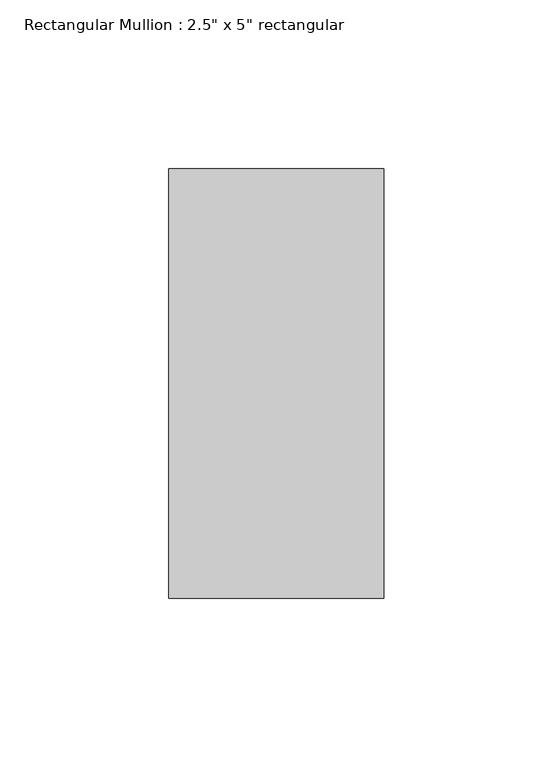
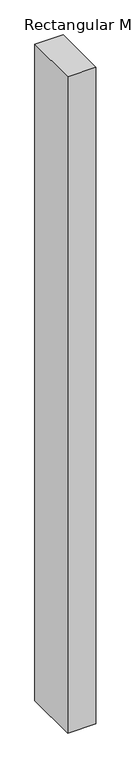
"""IFC4 building model written with IfcOpenShell, lengths in millimetres: member geometry."""

from ifc_helpers import new_model, si_unit, frame, origin, place, context, project, spatial, polyline, outline, extrude, source, transform, mapped, element, save


def member_6526e201(model_context):
    return source(origin(), model_context, "Body", "SweptSolid", [
        extrude(outline(polyline([(0.0, 63.5), (0.0, -63.5), (-63.5, -63.5), (-63.5, 63.5), (0.0, 63.5)])), frame((0.0, 0.0, -1556.4785779), z_axis=(0.0, 0.0, 1.0), x_axis=(1.0, 0.0, 0.0)), (0.0, 0.0, 1.0), 1556.4785779),
    ])


if __name__ == "__main__":
    model = new_model("IFC4")
    model_context = context("Model", 3, world=origin())
    ifc_project = project(units=[si_unit("LENGTHUNIT", "METRE", prefix="MILLI")], contexts=[model_context])
    site = spatial("IfcSite", under=ifc_project)
    building = spatial("IfcBuilding", under=site)
    placement = place(None, origin())
    member_shape = member_6526e201(model_context)
    element("IfcMember", 1, ObjectType="Rectangular Mullion : 2.5\" x 5\" rectangular", at=placement, inside=building, context=model_context, shape_type="MappedRepresentation", body=[
        mapped(member_shape, transform((0.0, 0.0, 0.0), x_axis=(1.0, 0.0, 0.0), y_axis=(0.0, 1.0, 0.0), z_axis=(0.0, 0.0, 1.0))),
    ])
    save(model, "model.ifc")

# Revit data of these elements
# Type "Rectangular Mullion : 2.5\" x 5\" rectangular"
#   built-in parameter 1007304 = 0.416667 (stored number, unit not read)
#   built-in parameter 1007301 = 0.104167 (stored number, unit not read)
#   built-in parameter 1007300 = 0.104167 (stored number, unit not read)
# Element 1 (IfcMember, "Rectangular Mullion : 2.5\" x 5\" rectangular")
#   Materials on its faces: "Aluminum"
# Materials
#   "Aluminum": class "Metal", colour RGB 247 247 247, transparency 0, Description = "Aluminum 6061", Cost = 0
